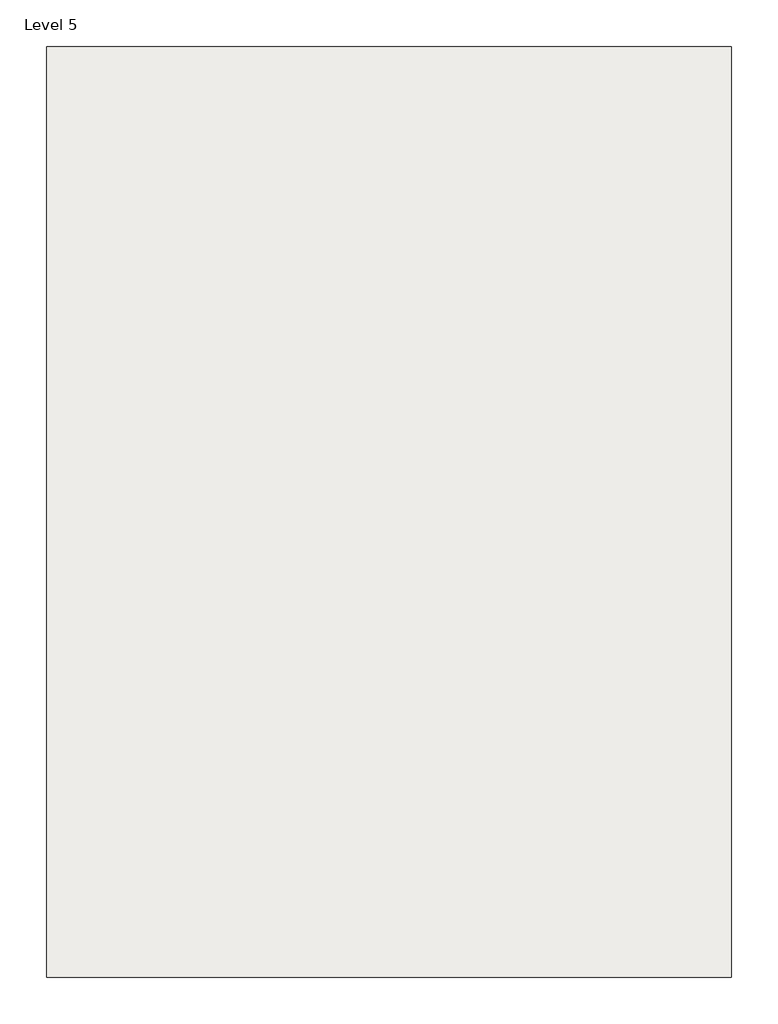
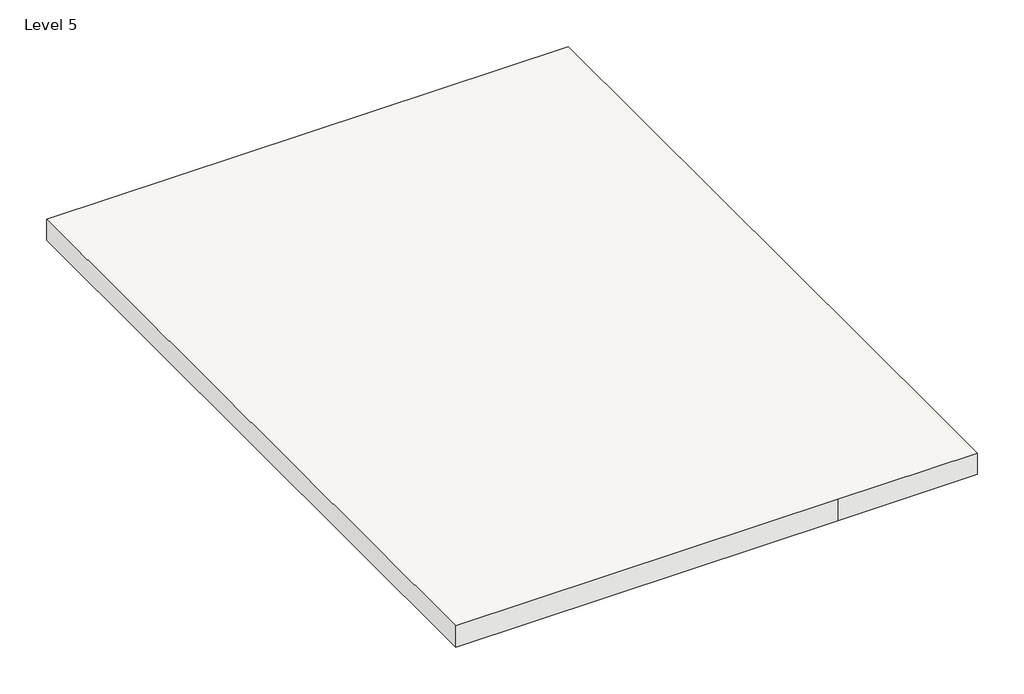
# One storey: 1 roof.
"""IFC4 building model written with IfcOpenShell, lengths in millimetres."""

from ifc_helpers import new_model, si_unit, frame, origin, place, context, project, spatial, polyline, outline, extrude, element, save

model = new_model("IFC4")

# Units and contexts
model_context = context("Model", 3, world=origin())
ifc_project = project(units=[si_unit("LENGTHUNIT", "METRE", prefix="MILLI")], contexts=[model_context])

# Site, building, storey
site = spatial("IfcSite", under=ifc_project)
building = spatial("IfcBuilding", under=site)
storey = spatial("IfcBuildingStorey", under=building, Name="Level 5", Elevation=14630.4)

# Roof
placement = place(None, origin())
element("IfcRoof", 1, ObjectType="Generic - 12\"", at=placement, inside=storey, context=model_context, shape_type="SweptSolid", body=[
    extrude(outline(polyline([(-9454.9432037, 10010.2548743), (-2342.9432037, 10010.2548743), (-2342.9432037, 1247.2548743), (-2342.9432037, 345.6498736), (-4247.9432037, 345.6498736), (-9454.9432037, 345.6498736), (-9454.9432037, 10010.2548743)])), frame((0.0, 0.0, 14630.4), z_axis=(0.0, 0.0, 1.0), x_axis=(1.0, 0.0, 0.0)), (0.0, 0.0, 1.0), 304.8),
])

save(model, "model.ifc")

# Revit data of these elements
# Type "Generic - 12\""
#   Assembly Code = "B1020"
#   Layers, outside or top first: 1' - 0" no material (function 1)
# Element 1 (IfcRoof, "Generic - 12\"")
#   built-in parameter 1001705 = 49 (stored number, unit not read)
#   built-in parameter 1001710 = 33615
#   Phase Created = New Construction
#   Materials on its faces: "Default Roof"
# Materials
#   "Default Roof": colour RGB 88 101 114, transparency 0
